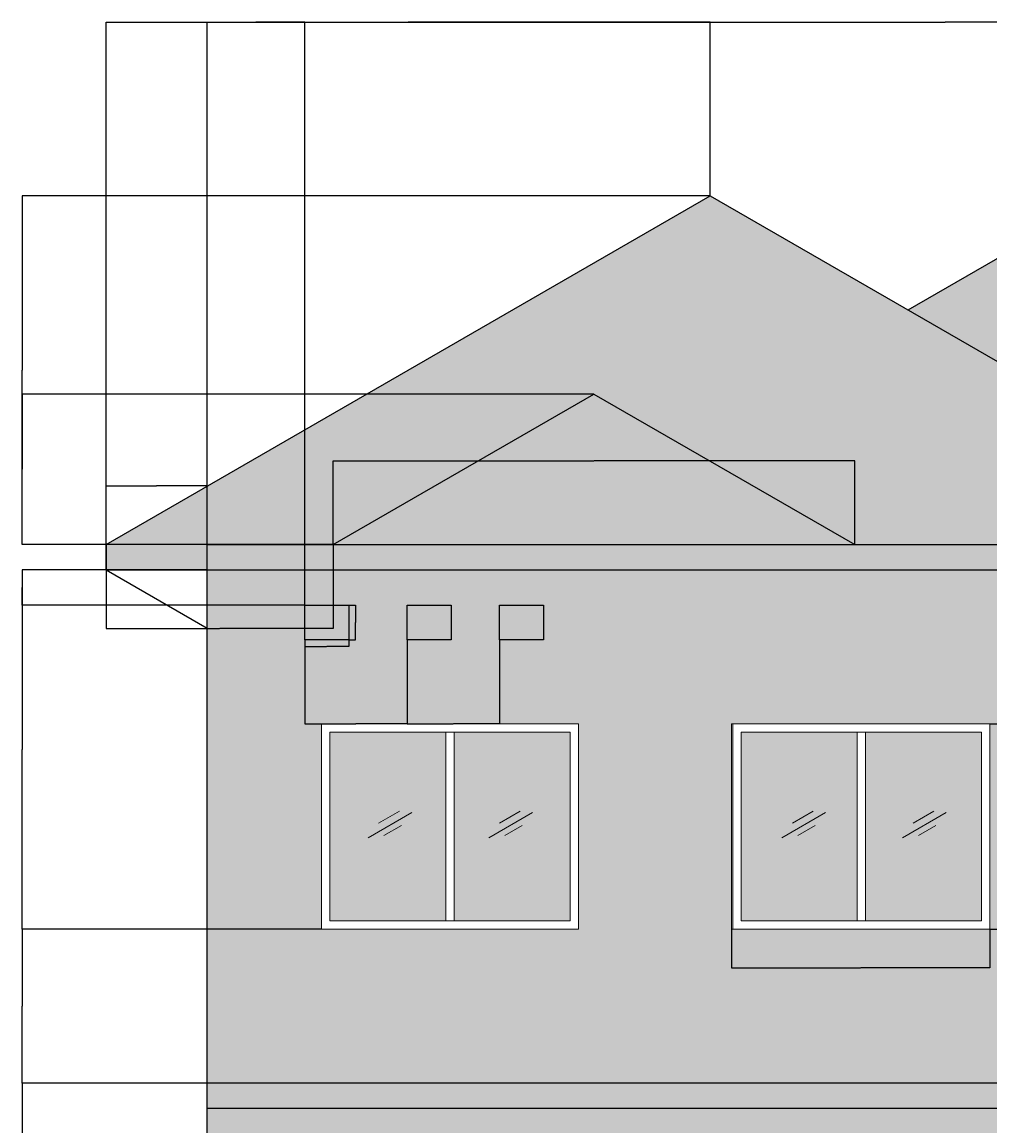
# Model space of a CAD drawing. Units: millimetres. Extents: x 2511 to 24632, y 2213 to 12972.
# Tile 4 of 5: x 13664 to 19414, y 6412 to 12972. Entities that reach past the tile are written whole.
import ezdxf

# ---------------------------------------------------------------- set-up
doc = ezdxf.new("R2010")
doc.units = ezdxf.units.MM
for name, color, linetype, lineweight in [('A-ANNO-DIMS', 2, 'Continuous', 18), ('A-ELEV', 7, 'Continuous', 25), ('A-ELEV-GLAZ', 7, 'Continuous', 18), ('A-ELEV-PATT', 13, 'Continuous', 9), ('A-ROOF', 7, 'Continuous', 25), ('A-ROOF-PATT', 13, 'Continuous', 13)]:
    doc.layers.add(name, color=color, linetype=linetype, lineweight=lineweight)
doc.layers.add('A-GLAZ-PATT', color=141, linetype='Continuous', lineweight=9, true_color=0xadddf7)
doc.styles.get("Standard").update_dxf_attribs({"font": 'arial.ttf'})
doc.dimstyles.get("Standard").update_dxf_attribs({"dimtxt": 0.18, "dimasz": 0.18, "dimexe": 0.18, "dimexo": 0.0625, "dimgap": 0.09, "dimtad": 0, "dimtih": 1, "dimtoh": 1, "dimdec": 4, "dimzin": 0, "dimdsep": 46, "dimtxsty": 'Standard', "dimcen": 0.09, "dimadec": 0, "dimazin": 0, "dimtfac": 1, "dimtdec": 4, "dimtofl": 0, "dimtmove": 0, "dimatfit": 3, "dimfxl": 1, "dimtolj": 1, "dimtzin": 0, "dimarcsym": 0})

# ---------------------------------------------------------------- blocks, each defined once
blk = doc.blocks.new('WINDOW-FRAME-1528-ELEV')
for p, q in [((3.45580574503e-05, -0.0004698816292148), (3.45580574503e-05, 1219.999530118371)), ((3.45580574503e-05, 1219.999530118371), (1527.988197152912, 1219.999530118371)), ((1527.988197152912, 1219.999530118371), (1527.988197152912, -0.0004698816292148)), ((738.9941158554847, 1169.999530118371), (738.9941158554847, 49.99953011837078)), ((788.9941158554847, 1169.999530118371), (788.9941158554847, 49.99953011837078)), ((1527.988197152912, -0.0004698816292148), (3.45580574503e-05, -0.0004698816292148))]:
    blk.add_line(p, q)
for points in [[(3.45580574503e-05, 1219.999530118371), (1527.988197152912, 1219.999530118371), (1527.988197152912, -0.0004698816292148), (3.45580574503e-05, -0.0004698816292148)], [(50.00003455805745, 1169.999530118371), (1477.988197152912, 1169.999530118371), (1477.988197152912, 49.99953011837078), (50.00003455805745, 49.99953011837078)]]:
    blk.add_lwpolyline(points, close=True)
blk = doc.blocks.new('WINDOW-FRAME-1536-ELEV')
for p, q in [((-0.0001940248657775, -0.0004698816292148), (-0.0001940248657775, 1219.999530118371)), ((-0.0001940248657775, 1219.999530118371), (1536.172544795805, 1219.999530118371)), ((1536.172544795805, 1219.999530118371), (1536.172544795805, -0.0004698816292148)), ((747.1784634983741, 1169.999530118371), (747.1784634983741, 49.99953011837078)), ((797.1784634983742, 1169.999530118371), (797.1784634983742, 49.99953011837078)), ((1536.172544795805, -0.0004698816292148), (-0.0001940248657775, -0.0004698816292148))]:
    blk.add_line(p, q)
for points in [[(8.184382200950495, 1219.999530118371), (1536.172544795805, 1219.999530118371), (1536.172544795805, -0.0004698816292148), (8.184382200950495, -0.0004698816292148)], [(58.1843822009505, 1169.999530118371), (1486.172544795805, 1169.999530118371), (1486.172544795805, 49.99953011837078), (58.1843822009505, 49.99953011837078)]]:
    blk.add_lwpolyline(points, close=True)
blk = doc.blocks.new('GLASS-REFLECTION')
for p, q in [((0.000348498528183, -0.0002333358270334), (259.2110812861792, 149.655153015964)), ((62.47510116635385, 86.0291626371336), (186.2553756901197, 157.4937374537958)), ((94.69077173755068, 13.20916119840785), (197.7341820365163, 72.70130187273116))]:
    blk.add_line(p, q)
blk = doc.blocks.new('FACADE-VENT-RECT')
blk.add_lwpolyline([(-0.0001923483068822, 206.5969172187779), (261.6107656867971, 206.5969172187779), (261.6107656867971, -0.0003445679158176), (-0.0001923483068822, -0.0003445679158176)], close=True)
blk = doc.blocks.new('*D23')
at = {"layer": 'A-ANNO-DIMS', "color": 0, "lineweight": -2, "transparency": 16777216}
for p, q in [((15342.91080765169, 9299.824155432085), (15342.91080765169, 9260.46501172682)), ((15343.09080765169, 9260.64501172682), (15472.74335351781, 9260.64501172682)), ((15604.34176568679, 9260.64501172682), (15474.68921982067, 9260.64501172682)), ((15604.52176568679, 9299.824155432085), (15604.52176568679, 9260.46501172682))]:
    blk.add_line(p, q, dxfattribs=at)
at = {"layer": 'A-ANNO-DIMS', "color": 0, "transparency": 16777216}
for points in [[(15343.09080765169, 9260.67501172682), (15343.09080765169, 9260.615011726817), (15342.91080765169, 9260.64501172682)], [(15604.34176568679, 9260.67501172682), (15604.34176568679, 9260.615011726817), (15604.52176568679, 9260.64501172682)]]:
    blk.add_solid(points, dxfattribs=at)
at = {"layer": 'Defpoints', "color": 0, "transparency": 16777216}
for p in [(15342.91080765169, 9299.886655432087), (15604.52176568679, 9299.886655432087), (15604.52176568679, 9260.64501172682)]:
    blk.add_point(p, dxfattribs=at)
at = {"layer": 'A-ANNO-DIMS', "color": 0, "transparency": 16777216, "insert": (15473.71628666924, 9260.64501172682), "char_height": 0.18, "attachment_point": 5}
blk.add_mtext('\\A1;VENT 262 TYP.', dxfattribs=at)
blk = doc.blocks.new('*D24')
at = {"layer": 'A-ANNO-DIMS', "color": 0, "lineweight": -2, "transparency": 16777216}
for p, q in [((15604.5842656868, 9506.483917218786), (15643.94340939208, 9506.483917218786)), ((15643.76340939207, 9506.303917218786), (15643.76340939207, 9403.367189463226)), ((15643.76340939207, 9300.066655432089), (15643.76340939207, 9403.003383187648)), ((15604.5842656868, 9299.886655432088), (15643.94340939208, 9299.886655432088))]:
    blk.add_line(p, q, dxfattribs=at)
at = {"layer": 'A-ANNO-DIMS', "color": 0, "transparency": 16777216}
for points in [[(15643.73340939208, 9506.303917218786), (15643.79340939208, 9506.303917218786), (15643.76340939207, 9506.483917218786)], [(15643.73340939208, 9300.066655432089), (15643.79340939208, 9300.066655432089), (15643.76340939207, 9299.886655432088)]]:
    blk.add_solid(points, dxfattribs=at)
at = {"layer": 'Defpoints', "color": 0, "transparency": 16777216}
for p in [(15604.5217656868, 9506.483917218786), (15643.76340939207, 9506.483917218786), (15604.5217656868, 9299.886655432088)]:
    blk.add_point(p, dxfattribs=at)
at = {"layer": 'A-ANNO-DIMS', "color": 0, "transparency": 16777216, "insert": (15643.76340939207, 9403.18528632543), "char_height": 0.18, "attachment_point": 5}
blk.add_mtext('\\A1;207 TYP.', dxfattribs=at)
blk = doc.blocks.new('*D33')
at = {"layer": 'A-ANNO-DIMS', "color": 0, "lineweight": -2, "transparency": 16777216}
for p, q in [((17877.81880597513, 7581.154030118369), (17877.81880597513, 7350.610619295268)), ((19413.9915447958, 7581.154030118369), (19413.9915447958, 7350.610619295268)), ((17877.99880597513, 7350.790619295269), (18644.76734455327, 7350.790619295269)), ((19413.8115447958, 7350.790619295269), (18647.04300621766, 7350.790619295269))]:
    blk.add_line(p, q, dxfattribs=at)
at = {"layer": 'A-ANNO-DIMS', "color": 0, "transparency": 16777216}
for points in [[(17877.99880597513, 7350.820619295268), (17877.99880597513, 7350.760619295269), (17877.81880597513, 7350.790619295269)], [(19413.8115447958, 7350.820619295268), (19413.8115447958, 7350.760619295269), (19413.9915447958, 7350.790619295269)]]:
    blk.add_solid(points, dxfattribs=at)
at = {"layer": 'Defpoints', "color": 0, "transparency": 16777216}
for p in [(17877.81880597513, 7581.21653011837), (19413.9915447958, 7581.21653011837), (19413.9915447958, 7350.790619295269)]:
    blk.add_point(p, dxfattribs=at)
at = {"layer": 'A-ANNO-DIMS', "color": 0, "transparency": 16777216, "insert": (18645.90517538547, 7350.790619295269), "char_height": 0.18, "attachment_point": 5}
blk.add_mtext('\\A1;FRAME 1536 TYP.', dxfattribs=at)
blk = doc.blocks.new('*D34')
at = {"layer": 'A-ANNO-DIMS', "color": 0, "lineweight": -2, "transparency": 16777216}
for p, q in [((19414.05404479581, 8801.216530118374), (19644.59745561891, 8801.216530118374)), ((19644.41745561891, 8801.036530118374), (19644.41745561892, 8191.398433256164)), ((19644.41745561892, 7581.396530118374), (19644.41745561892, 8191.034626980584)), ((19414.05404479581, 7581.216530118374), (19644.59745561892, 7581.216530118374))]:
    blk.add_line(p, q, dxfattribs=at)
at = {"layer": 'A-ANNO-DIMS', "color": 0, "transparency": 16777216}
for points in [[(19644.38745561891, 8801.036530118374), (19644.44745561891, 8801.036530118374), (19644.41745561891, 8801.216530118374)], [(19644.38745561892, 7581.396530118374), (19644.44745561891, 7581.396530118374), (19644.41745561892, 7581.216530118374)]]:
    blk.add_solid(points, dxfattribs=at)
at = {"layer": 'Defpoints', "color": 0, "transparency": 16777216}
for p in [(19413.99154479581, 8801.216530118374), (19644.41745561891, 8801.216530118374), (19413.99154479581, 7581.216530118374)]:
    blk.add_point(p, dxfattribs=at)
at = {"layer": 'A-ANNO-DIMS', "color": 0, "transparency": 16777216, "insert": (19644.41745561891, 8191.216530118365), "char_height": 0.18, "attachment_point": 5}
blk.add_mtext('\\A1;1220 TYP.', dxfattribs=at)
blk = doc.blocks.new('*D64')
at = {"layer": 'A-ANNO-DIMS', "color": 0, "lineweight": -2, "transparency": 16777216}
for p, q in [((14162.809797, 9866.279030000002), (14162.809797, 12971.685584)), ((14162.989797, 12971.505584), (19147.45133178854, 12971.505584)), ((24132.629797, 12971.505584), (19148.16826221146, 12971.505584)), ((24132.809797, 9716.27903), (24132.809797, 12971.685584))]:
    blk.add_line(p, q, dxfattribs=at)
at = {"layer": 'A-ANNO-DIMS', "color": 0, "transparency": 16777216}
for points in [[(14162.989797, 12971.535584), (14162.989797, 12971.475584), (14162.809797, 12971.505584)], [(24132.629797, 12971.535584), (24132.629797, 12971.475584), (24132.809797, 12971.505584)]]:
    blk.add_solid(points, dxfattribs=at)
at = {"layer": 'Defpoints', "color": 0, "transparency": 16777216}
for p in [(14162.809797, 12971.505584), (14162.809797, 9866.21653), (24132.809797, 9716.21653)]:
    blk.add_point(p, dxfattribs=at)
at = {"layer": 'A-ANNO-DIMS', "color": 0, "transparency": 16777216, "insert": (19147.809797, 12971.505584), "char_height": 0.18, "attachment_point": 5}
blk.add_mtext('\\A1;9970', dxfattribs=at)
blk = doc.blocks.new('*D68')
at = {"layer": 'A-ANNO-DIMS', "color": 0, "lineweight": -2, "transparency": 16777216}
for p, q in [((14762.747297, 6666.216530000004), (13663.87979700001, 6666.216530000003)), ((13664.05979700001, 6666.036530000003), (13664.05979700001, 5523.898433137791)), ((13664.05979700001, 4381.39653), (13664.05979700001, 5523.534626862211)), ((15441.75253500001, 4381.216530000002), (13663.87979700001, 4381.21653))]:
    blk.add_line(p, q, dxfattribs=at)
at = {"layer": 'A-ANNO-DIMS', "color": 0, "transparency": 16777216}
for points in [[(13664.02979700001, 6666.036530000003), (13664.08979700001, 6666.036530000003), (13664.05979700001, 6666.216530000003)], [(13664.02979700001, 4381.39653), (13664.08979700001, 4381.39653), (13664.05979700001, 4381.21653)]]:
    blk.add_solid(points, dxfattribs=at)
at = {"layer": 'Defpoints', "color": 0, "transparency": 16777216}
for p in [(13664.05979700001, 6666.216530000003), (14762.809797, 6666.216530000004), (15441.81503500001, 4381.216530000002)]:
    blk.add_point(p, dxfattribs=at)
at = {"layer": 'A-ANNO-DIMS', "color": 0, "transparency": 16777216, "insert": (13664.05979700001, 5523.716529999997), "char_height": 0.18, "attachment_point": 5}
blk.add_mtext('\\A1;2285', dxfattribs=at)
blk = doc.blocks.new('*D69')
at = {"layer": 'A-ANNO-DIMS', "color": 0, "lineweight": -2, "transparency": 16777216}
for p, q in [((15441.75253500001, 7581.216530000003), (13663.87979700001, 7581.216530000003)), ((13664.05979700001, 7581.036530000003), (13664.05979700001, 7123.898433137792)), ((13664.05979700001, 6666.396530000003), (13664.05979700001, 7123.534626862213)), ((14762.747297, 6666.216530000004), (13663.87979700001, 6666.216530000003))]:
    blk.add_line(p, q, dxfattribs=at)
at = {"layer": 'A-ANNO-DIMS', "color": 0, "transparency": 16777216}
for points in [[(13664.02979700001, 7581.036530000003), (13664.08979700001, 7581.036530000003), (13664.05979700001, 7581.216530000003)], [(13664.02979700001, 6666.396530000003), (13664.08979700001, 6666.396530000003), (13664.05979700001, 6666.216530000003)]]:
    blk.add_solid(points, dxfattribs=at)
at = {"layer": 'Defpoints', "color": 0, "transparency": 16777216}
for p in [(13664.05979700001, 7581.216530000003), (15441.81503500001, 7581.216530000003), (14762.809797, 6666.216530000004)]:
    blk.add_point(p, dxfattribs=at)
at = {"layer": 'A-ANNO-DIMS', "color": 0, "transparency": 16777216, "insert": (13664.05979700001, 7123.716529999997), "char_height": 0.18, "attachment_point": 5}
blk.add_mtext('\\A1;915', dxfattribs=at)
blk = doc.blocks.new('*D70')
at = {"layer": 'A-ANNO-DIMS', "color": 0, "lineweight": -2, "transparency": 16777216}
for p, q in [((14762.747297, 9716.216530000003), (13663.87979700001, 9716.216530000003)), ((13664.05979700001, 9716.036530000003), (13664.05979700001, 8648.898494529332)), ((13664.05979700001, 7581.396530000003), (13664.05979700001, 8648.534565470674)), ((15441.75253500001, 7581.216530000003), (13663.87979700001, 7581.216530000003))]:
    blk.add_line(p, q, dxfattribs=at)
at = {"layer": 'A-ANNO-DIMS', "color": 0, "transparency": 16777216}
for points in [[(13664.02979700001, 9716.036530000003), (13664.08979700001, 9716.036530000003), (13664.05979700001, 9716.216530000003)], [(13664.02979700001, 7581.396530000003), (13664.08979700001, 7581.396530000003), (13664.05979700001, 7581.216530000003)]]:
    blk.add_solid(points, dxfattribs=at)
at = {"layer": 'Defpoints', "color": 0, "transparency": 16777216}
for p in [(13664.05979700001, 9716.216530000003), (14762.809797, 9716.216530000003), (15441.81503500001, 7581.216530000003)]:
    blk.add_point(p, dxfattribs=at)
at = {"layer": 'A-ANNO-DIMS', "color": 0, "transparency": 16777216, "insert": (13664.05979700001, 8648.71653), "char_height": 0.18, "attachment_point": 5}
blk.add_mtext('\\A1;2135', dxfattribs=at)
blk = doc.blocks.new('*D82')
at = {"layer": 'A-ANNO-DIMS', "color": 0, "lineweight": -2, "transparency": 16777216}
for p, q in [((14162.809797, 9716.27903), (14162.809797, 10215.14653)), ((14162.989797, 10214.96653), (14462.5207656221, 10214.96653)), ((14762.629797, 10214.96653), (14463.0988283779, 10214.96653)), ((14762.809797, 9716.27903), (14762.809797, 10215.14653))]:
    blk.add_line(p, q, dxfattribs=at)
at = {"layer": 'A-ANNO-DIMS', "color": 0, "transparency": 16777216}
for points in [[(14162.989797, 10214.99653), (14162.989797, 10214.93653), (14162.809797, 10214.96653)], [(14762.629797, 10214.99653), (14762.629797, 10214.93653), (14762.809797, 10214.96653)]]:
    blk.add_solid(points, dxfattribs=at)
at = {"layer": 'Defpoints', "color": 0, "transparency": 16777216}
for p in [(14762.809797, 10214.96653), (14162.809797, 9716.21653), (14762.809797, 9716.21653)]:
    blk.add_point(p, dxfattribs=at)
at = {"layer": 'A-ANNO-DIMS', "color": 0, "transparency": 16777216, "insert": (14462.809797, 10214.96653), "char_height": 0.18, "attachment_point": 5}
blk.add_mtext('\\A1;600', dxfattribs=at)
blk = doc.blocks.new('*D84')
at = {"layer": 'A-ANNO-DIMS', "color": 0, "lineweight": -2, "transparency": 16777216}
for p, q in [((15950.742303, 9299.824155), (15950.742303, 8800.956655)), ((16500.795593, 9299.824155), (16500.795593, 8800.956655)), ((15950.922303, 8801.136655), (16225.48040775443, 8801.136655)), ((16500.615593, 8801.136655), (16226.05748824557, 8801.136655))]:
    blk.add_line(p, q, dxfattribs=at)
at = {"layer": 'A-ANNO-DIMS', "color": 0, "transparency": 16777216}
for points in [[(15950.922303, 8801.166655), (15950.922303, 8801.106655), (15950.742303, 8801.136655)], [(16500.615593, 8801.166655), (16500.615593, 8801.106655), (16500.795593, 8801.136655)]]:
    blk.add_solid(points, dxfattribs=at)
at = {"layer": 'Defpoints', "color": 0, "transparency": 16777216}
for p in [(15950.742303, 9299.886654999998), (16500.795593, 9299.886654999998), (15950.742303, 8801.136655)]:
    blk.add_point(p, dxfattribs=at)
at = {"layer": 'A-ANNO-DIMS', "color": 0, "transparency": 16777216, "insert": (16225.768948, 8801.136655), "char_height": 0.18, "attachment_point": 5}
blk.add_mtext('\\A1;550', dxfattribs=at)
blk = doc.blocks.new('*D85')
at = {"layer": 'A-ANNO-DIMS', "color": 0, "lineweight": -2, "transparency": 16777216}
for p, q in [((15342.910808, 9299.824155), (15342.910808, 8800.956655)), ((15950.742303, 9299.824155), (15950.742303, 8800.956655)), ((15343.090808, 8801.136655), (15646.4321762367, 8801.136655)), ((15950.562303, 8801.136655), (15647.2209347633, 8801.136655))]:
    blk.add_line(p, q, dxfattribs=at)
at = {"layer": 'A-ANNO-DIMS', "color": 0, "transparency": 16777216}
for points in [[(15343.090808, 8801.166655), (15343.090808, 8801.106655), (15342.910808, 8801.136655)], [(15950.562303, 8801.166655), (15950.562303, 8801.106655), (15950.742303, 8801.136655)]]:
    blk.add_solid(points, dxfattribs=at)
at = {"layer": 'Defpoints', "color": 0, "transparency": 16777216}
for p in [(15342.910808, 9299.886654999998), (15950.742303, 9299.886654999998), (15342.910808, 8801.136655)]:
    blk.add_point(p, dxfattribs=at)
at = {"layer": 'A-ANNO-DIMS', "color": 0, "transparency": 16777216, "insert": (15646.8265555, 8801.136655), "char_height": 0.18, "attachment_point": 5}
blk.add_mtext('\\A1;607.8', dxfattribs=at)
blk = doc.blocks.new('*D86')
at = {"layer": 'A-ANNO-DIMS', "color": 0, "lineweight": -2, "transparency": 16777216}
for p, q in [((14762.809797, 9716.27903), (14762.809797, 12971.685584)), ((14762.989797, 12971.505584), (15052.48397234993, 12971.505584)), ((15342.730808, 12971.505584), (15053.23663265007, 12971.505584)), ((15342.910808, 9506.546417), (15342.910808, 12971.685584))]:
    blk.add_line(p, q, dxfattribs=at)
at = {"layer": 'A-ANNO-DIMS', "color": 0, "transparency": 16777216}
for points in [[(14762.989797, 12971.535584), (14762.989797, 12971.475584), (14762.809797, 12971.505584)], [(15342.730808, 12971.535584), (15342.730808, 12971.475584), (15342.910808, 12971.505584)]]:
    blk.add_solid(points, dxfattribs=at)
at = {"layer": 'Defpoints', "color": 0, "transparency": 16777216}
for p in [(15342.910808, 12971.505584), (14762.809797, 9716.21653), (15342.910808, 9506.483917)]:
    blk.add_point(p, dxfattribs=at)
at = {"layer": 'A-ANNO-DIMS', "color": 0, "transparency": 16777216, "insert": (15052.8603025, 12971.505584), "char_height": 0.18, "attachment_point": 5}
blk.add_mtext('\\A1;580.1', dxfattribs=at)
blk = doc.blocks.new('*D87')
at = {"layer": 'A-ANNO-DIMS', "color": 0, "lineweight": -2, "transparency": 16777216}
for p, q in [((14762.747297, 9716.216530000003), (13663.87979700001, 9716.216530000003)), ((13664.05979700001, 9716.036530000003), (13664.05979700001, 9611.532188029334)), ((13664.05979700001, 9506.663917000002), (13664.05979700001, 9611.168258970672)), ((15342.848308, 9506.483917000001), (13663.87979700001, 9506.483917000001))]:
    blk.add_line(p, q, dxfattribs=at)
at = {"layer": 'A-ANNO-DIMS', "color": 0, "transparency": 16777216}
for points in [[(13664.02979700001, 9716.036530000003), (13664.08979700001, 9716.036530000003), (13664.05979700001, 9716.216530000003)], [(13664.02979700001, 9506.663917000002), (13664.08979700001, 9506.663917000002), (13664.05979700001, 9506.483917000001)]]:
    blk.add_solid(points, dxfattribs=at)
at = {"layer": 'Defpoints', "color": 0, "transparency": 16777216}
for p in [(14762.809797, 9716.216530000003), (13664.05979700001, 9506.483917000001), (15342.910808, 9506.483917000001)]:
    blk.add_point(p, dxfattribs=at)
at = {"layer": 'A-ANNO-DIMS', "color": 0, "transparency": 16777216, "insert": (13664.05979700001, 9611.350223499998), "char_height": 0.18, "attachment_point": 5}
blk.add_mtext('\\A1;209.73', dxfattribs=at)
blk = doc.blocks.new('*D88')
at = {"layer": 'A-ANNO-DIMS', "color": 0, "lineweight": -2, "transparency": 16777216}
for p, q in [((17752.200329, 11938.588205), (13663.87979700001, 11938.588205)), ((13664.05979700001, 11938.408205), (13664.05979700001, 10902.58427063779)), ((13664.05979700001, 9866.396530000004), (13664.05979700001, 10902.22046436221)), ((14162.747297, 9866.216530000003), (13663.87979700001, 9866.216530000003))]:
    blk.add_line(p, q, dxfattribs=at)
at = {"layer": 'A-ANNO-DIMS', "color": 0, "transparency": 16777216}
for points in [[(13664.02979700001, 11938.408205), (13664.08979700001, 11938.408205), (13664.05979700001, 11938.588205)], [(13664.02979700001, 9866.396530000004), (13664.08979700001, 9866.396530000004), (13664.05979700001, 9866.216530000003)]]:
    blk.add_solid(points, dxfattribs=at)
at = {"layer": 'Defpoints', "color": 0, "transparency": 16777216}
for p in [(13664.05979700001, 11938.588205), (17752.262829, 11938.588205), (14162.80979700001, 9866.216530000003)]:
    blk.add_point(p, dxfattribs=at)
at = {"layer": 'A-ANNO-DIMS', "color": 0, "transparency": 16777216, "insert": (13664.05979700001, 10902.4023675), "char_height": 0.18, "attachment_point": 5}
blk.add_mtext('\\A1;2072.4', dxfattribs=at)
blk = doc.blocks.new('*D90')
at = {"layer": 'A-ANNO-DIMS', "color": 0, "lineweight": -2, "transparency": 16777216}
for p, q in [((14162.809797, 9866.279030000002), (14162.809797, 12971.685584)), ((14162.989797, 12971.505584), (15957.07207016235, 12971.505584)), ((17752.082829, 12971.505584), (15958.00055583765, 12971.505584)), ((17752.262829, 11938.650705), (17752.262829, 12971.685584))]:
    blk.add_line(p, q, dxfattribs=at)
at = {"layer": 'A-ANNO-DIMS', "color": 0, "transparency": 16777216}
for points in [[(14162.989797, 12971.535584), (14162.989797, 12971.475584), (14162.809797, 12971.505584)], [(17752.082829, 12971.535584), (17752.082829, 12971.475584), (17752.262829, 12971.505584)]]:
    blk.add_solid(points, dxfattribs=at)
at = {"layer": 'Defpoints', "color": 0, "transparency": 16777216}
for p in [(17752.262829, 12971.505584), (17752.262829, 11938.588205), (14162.809797, 9866.21653)]:
    blk.add_point(p, dxfattribs=at)
at = {"layer": 'A-ANNO-DIMS', "color": 0, "transparency": 16777216, "insert": (15957.536313, 12971.505584), "char_height": 0.18, "attachment_point": 5}
blk.add_mtext('\\A1;3589.5', dxfattribs=at)
blk = doc.blocks.new('*D91')
at = {"layer": 'A-ANNO-DIMS', "color": 0, "lineweight": -2, "transparency": 16777216}
for p, q in [((15511.626108, 9866.279030000002), (15511.626108, 10365.14653)), ((18611.109928, 9866.279030000002), (18611.109928, 10365.14653)), ((15511.806108, 10364.96653), (17060.90377516235, 10364.96653)), ((18610.929928, 10364.96653), (17061.83226083765, 10364.96653))]:
    blk.add_line(p, q, dxfattribs=at)
at = {"layer": 'A-ANNO-DIMS', "color": 0, "transparency": 16777216}
for points in [[(15511.806108, 10364.99653), (15511.806108, 10364.93653), (15511.626108, 10364.96653)], [(18610.929928, 10364.99653), (18610.929928, 10364.93653), (18611.109928, 10364.96653)]]:
    blk.add_solid(points, dxfattribs=at)
at = {"layer": 'Defpoints', "color": 0, "transparency": 16777216}
for p in [(18611.109928, 10364.96653), (15511.626108, 9866.21653), (18611.109928, 9866.21653)]:
    blk.add_point(p, dxfattribs=at)
at = {"layer": 'A-ANNO-DIMS', "color": 0, "transparency": 16777216, "insert": (17061.368018, 10364.96653), "char_height": 0.18, "attachment_point": 5}
blk.add_mtext('\\A1;3099.5', dxfattribs=at)
blk = doc.blocks.new('*D92')
at = {"layer": 'A-ANNO-DIMS', "color": 0, "lineweight": -2, "transparency": 16777216}
for p, q in [((14162.809797, 9866.15403), (14162.809797, 9367.28653)), ((15511.626108, 9866.15403), (15511.626108, 9367.28653)), ((14162.989797, 9367.46653), (14836.76261143588, 9367.46653)), ((15511.446108, 9367.46653), (14837.67329356412, 9367.46653))]:
    blk.add_line(p, q, dxfattribs=at)
at = {"layer": 'A-ANNO-DIMS', "color": 0, "transparency": 16777216}
for points in [[(14162.989797, 9367.496530000002), (14162.989797, 9367.436529999999), (14162.809797, 9367.46653)], [(15511.446108, 9367.496530000002), (15511.446108, 9367.436529999999), (15511.626108, 9367.46653)]]:
    blk.add_solid(points, dxfattribs=at)
at = {"layer": 'Defpoints', "color": 0, "transparency": 16777216}
for p in [(14162.809797, 9866.21653), (15511.626108, 9866.21653), (14162.809797, 9367.46653)]:
    blk.add_point(p, dxfattribs=at)
at = {"layer": 'A-ANNO-DIMS', "color": 0, "transparency": 16777216, "insert": (14837.2179525, 9367.46653), "char_height": 0.18, "attachment_point": 5}
blk.add_mtext('\\A1;1348.8', dxfattribs=at)
blk = doc.blocks.new('*D93')
at = {"layer": 'A-ANNO-DIMS', "color": 0, "lineweight": -2, "transparency": 16777216}
for p, q in [((17061.30551800001, 10760.960439), (13663.87979700001, 10760.960439)), ((13664.05979700001, 10760.780439), (13664.05979700001, 10313.77038763779)), ((13664.05979700001, 9866.396530000004), (13664.05979700001, 10313.40658136221)), ((15511.56360800001, 9866.216530000003), (13663.87979700001, 9866.216530000003))]:
    blk.add_line(p, q, dxfattribs=at)
at = {"layer": 'A-ANNO-DIMS', "color": 0, "transparency": 16777216}
for points in [[(13664.02979700001, 10760.780439), (13664.08979700001, 10760.780439), (13664.05979700001, 10760.960439)], [(13664.02979700001, 9866.396530000004), (13664.08979700001, 9866.396530000004), (13664.05979700001, 9866.216530000003)]]:
    blk.add_solid(points, dxfattribs=at)
at = {"layer": 'Defpoints', "color": 0, "transparency": 16777216}
for p in [(17061.36801800001, 10760.960439), (13664.05979700001, 9866.216530000003), (15511.626108, 9866.216530000003)]:
    blk.add_point(p, dxfattribs=at)
at = {"layer": 'A-ANNO-DIMS', "color": 0, "transparency": 16777216, "insert": (13664.05979700001, 10313.5884845), "char_height": 0.18, "attachment_point": 5}
blk.add_mtext('\\A1;894.7', dxfattribs=at)

msp = doc.modelspace()

# ---------------------------------------------------------------- hatches: boundary and pattern name
at = {"layer": 'A-ELEV-PATT', "transparency": 33554551}
h = msp.add_hatch(color=256, dxfattribs=at)
h.dxf.hatch_style = 1
h.paths.add_polyline_path([(20858.80979657499, 6516.216530118374), (14762.80979657499, 6516.21653011837), (14762.80979657499, 3466.216530118371), (19843.80979657499, 3466.216530118371), (19843.80979657499, 5601.216530118371), (20718.80979657499, 5601.216530118371), (20718.80979657499, 3466.216530118371), (20858.80979657499, 3466.216530118371)])
h.paths.add_polyline_path([(16969.80319715291, 5601.216530118371), (16969.80319715291, 4381.21653011837), (15441.81503455806, 4381.21653011837), (15441.81503455806, 5601.216530118371)], flags=16)
h.paths.add_polyline_path([(16919.80319715291, 5551.21653011837), (16919.80319715291, 4431.21653011837), (15491.81503455806, 4431.21653011837), (15491.81503455806, 5551.21653011837)], flags=0)
h.paths.add_polyline_path([(17877.81880597513, 5601.216530118371), (19413.9915447958, 5601.216530118371), (19413.9915447958, 4381.21653011837), (17886.00338220095, 4381.21653011837), (17877.81880597513, 4381.21653011837)], flags=16)
h.paths.add_polyline_path([(17936.00338220095, 5551.21653011837), (19363.9915447958, 5551.21653011837), (19363.9915447958, 4431.21653011837), (17936.00338220095, 4431.21653011837)], flags=0)
h.paths.add_polyline_path([(20858.80979657499, 9716.216530118376), (14762.80979657499, 9716.21653011837), (14762.80979657499, 6666.21653011837), (19522.169078361, 6666.21653011837), (19522.169078361, 7733.216530118371), (20858.80979657499, 7733.216530118371)])
h.paths.add_polyline_path([(16969.80319715291, 8801.21653011837), (16969.80319715291, 7581.216530118371), (15441.81503455806, 7581.216530118371), (15441.81503455806, 8801.21653011837)], flags=16)
h.paths.add_polyline_path([(16919.80319715291, 8751.216530118369), (16919.80319715291, 7631.216530118371), (15491.81503455806, 7631.216530118371), (15491.81503455806, 8751.216530118369)], flags=0)
h.paths.add_polyline_path([(17877.81880597514, 8801.21653011837), (19413.9915447958, 8801.21653011837), (19413.9915447958, 7581.216530118371), (17886.00338220095, 7581.216530118371), (17877.81880597513, 7581.216530118371)], flags=16)
h.paths.add_polyline_path([(17936.00338220095, 8751.216530118369), (19363.9915447958, 8751.216530118369), (19363.9915447958, 7631.216530118371), (17936.00338220095, 7631.216530118371)], flags=0)
h.paths.add_polyline_path([(23051.60643531334, 9716.216530118376), (20858.80979657499, 9716.21653011837), (20858.80979657499, 7733.216530118371), (23051.60643531334, 7733.216530118371)])
h.paths.add_polyline_path([(23051.60643531335, 6516.216530118374), (20858.80979657499, 6516.216530118374), (20858.80979657499, 3516.21653011837), (23051.60643531335, 3516.21653011837)])
h = msp.add_hatch(color=256, dxfattribs=at)
h.dxf.hatch_style = 1
h.paths.add_polyline_path([(23708.80979657499, 6666.21653011837), (14762.80979657499, 6666.21653011837), (14762.80979657499, 6516.21653011837), (23708.80979657499, 6516.216530118374)])
at = {"layer": 'A-GLAZ-PATT'}
h = msp.add_hatch(color=256, dxfattribs=at)
h.dxf.hatch_style = 1
h.paths.add_polyline_path([(16180.80911585549, 8751.216530118369), (15491.81503455806, 8751.216530118369), (15491.81503455806, 7631.216530118371), (16180.80911585549, 7631.216530118371)])
h.paths.add_polyline_path([(16919.80319715291, 8751.216530118369), (16230.80911585548, 8751.216530118369), (16230.80911585548, 7631.216530118371), (16919.80319715291, 7631.216530118371)])
h.paths.add_polyline_path([(18624.99746349838, 8751.216530118369), (17936.00338220095, 8751.216530118369), (17936.00338220095, 7631.216530118371), (18624.99746349838, 7631.216530118371)])
h.paths.add_polyline_path([(19363.9915447958, 8751.216530118369), (18674.99746349837, 8751.216530118369), (18674.99746349837, 7631.216530118371), (19363.9915447958, 7631.216530118371)])
h.paths.add_polyline_path([(16180.80911585548, 5551.21653011837), (15491.81503455806, 5551.21653011837), (15491.81503455806, 4431.21653011837), (16180.80911585548, 4431.21653011837)])
h.paths.add_polyline_path([(16919.80319715291, 5551.21653011837), (16230.80911585548, 5551.21653011837), (16230.80911585548, 4431.21653011837), (16919.80319715291, 4431.21653011837)])
h.paths.add_polyline_path([(18624.99746349837, 5551.21653011837), (17936.00338220095, 5551.21653011837), (17936.00338220095, 4431.21653011837), (18624.99746349837, 4431.21653011837)])
h.paths.add_polyline_path([(19363.9915447958, 5551.21653011837), (18674.99746349837, 5551.21653011837), (18674.99746349837, 4431.21653011837), (19363.9915447958, 4431.21653011837)])
at = {"layer": 'A-ROOF-PATT'}
h = msp.add_hatch(dxfattribs=at)
h.set_pattern_fill('ANGLE', color=256, scale=15)
h.set_pattern_definition([(0, (11792.595132882, -12295.09862892571), (0, 104.775), [76.2, -28.575]), (90, (11792.595132882, -12295.09862892571), (-104.775, 6.4e-15), [76.2, -28.575])])
h.paths.add_polyline_path([(17752.26282908254, 11938.58820468012), (14162.80979657499, 9866.216530118376), (14762.80979657499, 9866.216530118376), (15511.62610781541, 9866.216530118376), (17061.36801812783, 10760.96043921169), (18611.10992844025, 9866.216530118376), (21341.71586159009, 9866.21653011837)])
h.paths.add_polyline_path([(21026.45751448832, 12472.755584324), (18926.75765114087, 11260.49330300292), (21341.71586159008, 9866.21653011837), (23532.80979657499, 9866.21653011837), (24132.80979657499, 9866.21653011837)])
h.paths.add_polyline_path([(17061.36801812783, 10760.96043921169), (15511.62610781541, 9866.216530118376), (18611.10992844025, 9866.21653011837)], flags=17)
at = {"layer": 'A-ROOF-PATT', "transparency": 33554551}
h = msp.add_hatch(color=256, dxfattribs=at)
h.dxf.hatch_style = 1
h.paths.add_polyline_path([(24132.80979657499, 9866.21653011837), (23532.80979657499, 9866.21653011837), (14762.80979657499, 9866.216530118376), (14162.80979657499, 9866.216530118376), (14162.80979657499, 9716.21653011837), (14762.80979657499, 9716.21653011837), (23532.80979657499, 9716.216530118376), (24132.80979657499, 9716.216530118376)])

# ---------------------------------------------------------------- linework, layer by layer
at = {"layer": 'A-ELEV'}
for p, q in [((14762.80979657499, 6666.21653011837), (14762.80979657499, 9716.216530118376)), ((14762.80979657499, 3466.216530118371), (14762.80979657499, 7733.216530118371)), ((23708.80979657499, 6666.21653011837), (14762.80979657499, 6666.21653011837)), ((14762.80979657499, 6516.21653011837), (23708.80979657499, 6516.216530118374))]:
    msp.add_line(p, q, dxfattribs=at)
at = {"layer": 'A-ROOF'}
for p, q in [((21026.45751448832, 12472.755584324), (18926.75765114087, 11260.49330300292)), ((14162.80979657499, 9866.216530118376), (17752.26282908254, 11938.58820468012)), ((17752.26282908254, 11938.58820468012), (21341.71586159009, 9866.21653011837)), ((15511.62610781541, 9866.216530118376), (17061.36801812783, 10760.96043921169)), ((17061.36801812783, 10760.96043921169), (18611.10992844024, 9866.216530118376)), ((14762.80979657499, 9866.216530118376), (14162.80979657499, 9866.216530118376)), ((14162.80979657499, 9866.216530118376), (14162.80979657499, 9716.21653011837)), ((14762.80979657499, 9866.216530118376), (23532.80979657499, 9866.21653011837)), ((14162.80979657499, 9716.21653011837), (14762.80979657499, 9716.21653011837)), ((14162.80979657499, 9716.21653011837), (14762.80979657499, 9369.806368604599)), ((14762.80979657499, 9716.21653011837), (23532.80979657499, 9716.216530118376))]:
    msp.add_line(p, q, dxfattribs=at)

# ---------------------------------------------------------------- block references
at = {"layer": 'A-ELEV'}
for p in [(15342.911, 9299.887), (15950.74249530715, 9299.887), (16500.79578584541, 9299.887)]:
    msp.add_blockref('FACADE-VENT-RECT', p, dxfattribs=at)
at = {"layer": 'A-ELEV-GLAZ'}
for name, p in [('WINDOW-FRAME-1528-ELEV', (15441.815, 7581.216999999999)), ('WINDOW-FRAME-1536-ELEV', (17877.819, 7581.216999999999)), ('GLASS-REFLECTION', (15719.254, 8124.306999999999)), ('GLASS-REFLECTION', (16437.39000946567, 8124.306999999999)), ('GLASS-REFLECTION', (18178.49078937554, 8124.306999999999)), ('GLASS-REFLECTION', (18894.90375053235, 8124.306999999999))]:
    msp.add_blockref(name, p, dxfattribs=at)

# ---------------------------------------------------------------- dimensions: what is measured, and where the dimension line sits
at = {"layer": 'A-ANNO-DIMS'}
for base, p1, p2, override, picture, middle in [((14162.809797, 12971.505584), (24132.809797, 9716.21653), (14162.809797, 9866.21653), {"dimdec": 0, "dimlfac": 1, "dimrnd": 0, "dimzin": 0, "dimdsep": 46, "dimlunit": 2}, '*D64', (19147.809797, 12971.505584)), ((17752.262829, 12971.505584), (14162.809797, 9866.21653), (17752.262829, 11938.588205), {"dimdec": 1, "dimlfac": 1, "dimrnd": 0, "dimzin": 0, "dimdsep": 46, "dimlunit": 2}, '*D90', (15957.536313, 12971.505584)), ((15342.910808, 12971.505584), (14762.809797, 9716.21653), (15342.910808, 9506.483917), {"dimdec": 1, "dimlfac": 1, "dimrnd": 0, "dimzin": 0, "dimdsep": 46, "dimlunit": 2}, '*D86', (15052.8603025, 12971.505584)), ((18611.109928, 10364.96653), (15511.626108, 9866.21653), (18611.109928, 9866.21653), {"dimdec": 1, "dimlfac": 1, "dimrnd": 0, "dimzin": 0, "dimdsep": 46, "dimlunit": 2}, '*D91', (17061.368018, 10364.96653)), ((14762.809797, 10214.96653), (14162.809797, 9716.21653), (14762.809797, 9716.21653), {"dimdec": 0, "dimlfac": 1, "dimrnd": 0, "dimzin": 0, "dimdsep": 46, "dimlunit": 2}, '*D82', (14462.809797, 10214.96653))]:
    dim = msp.add_linear_dim(base=base, p1=p1, p2=p2, dimstyle='Standard', override=override, dxfattribs=at)
    dim.commit()
    dim.dimension.update_dxf_attribs({"geometry": picture, "text_midpoint": middle})
for base, p1, p2, angle, override, picture, middle in [((13664.05979700001, 11938.588205), (14162.809797, 9866.21653), (17752.262829, 11938.588205), 90, {"dimdec": 1, "dimlfac": 1, "dimrnd": 0, "dimzin": 0, "dimdsep": 46, "dimlunit": 2}, '*D88', (13664.05979700001, 10902.4023675)), ((13664.05979700001, 9866.216530000003), (17061.368018, 10760.960439), (15511.626108, 9866.21653), 90, {"dimdec": 1, "dimlfac": 1, "dimrnd": 0, "dimzin": 0, "dimdsep": 46, "dimlunit": 2}, '*D93', (13664.05979700001, 10313.5884845)), ((14162.809797, 9367.46653), (15511.626108, 9866.21653), (14162.809797, 9866.21653), 180, {"dimdec": 1, "dimlfac": 1, "dimrnd": 0, "dimzin": 0, "dimdsep": 46, "dimlunit": 2}, '*D92', (14837.2179525, 9367.46653)), ((13664.05979700001, 9506.483917000001), (14762.809797, 9716.21653), (15342.910808, 9506.483917), 90, {"dimdec": 2, "dimlfac": 1, "dimrnd": 0, "dimzin": 0, "dimdsep": 46, "dimlunit": 2}, '*D87', (13664.05979700001, 9611.350223499998)), ((13664.05979700001, 9716.216530000003), (15441.815035, 7581.21653), (14762.809797, 9716.21653), 90, {"dimdec": 0, "dimlfac": 1, "dimrnd": 0, "dimzin": 0, "dimdsep": 46, "dimlunit": 2}, '*D70', (13664.05979700001, 8648.71653)), ((15342.910808, 8801.136655), (15950.742303, 9299.886654999998), (15342.910808, 9299.886654999998), 180, {"dimdec": 1, "dimlfac": 1, "dimrnd": 0, "dimzin": 0, "dimdsep": 46, "dimlunit": 2}, '*D85', (15646.8265555, 8801.136655)), ((15950.742303, 8801.136655), (16500.795593, 9299.886654999998), (15950.742303, 9299.886654999998), 180, {"dimdec": 0, "dimlfac": 1, "dimrnd": 0, "dimzin": 0, "dimdsep": 46, "dimlunit": 2}, '*D84', (16225.768948, 8801.136655)), ((13664.05979700001, 7581.216530000003), (14762.809797, 6666.216529999999), (15441.815035, 7581.21653), 90, {"dimdec": 0, "dimlfac": 1, "dimrnd": 0, "dimzin": 0, "dimdsep": 46, "dimlunit": 2}, '*D69', (13664.05979700001, 7123.716529999997)), ((13664.05979700001, 6666.216530000003), (15441.815035, 4381.216529999999), (14762.809797, 6666.216529999999), 90, {"dimdec": 0, "dimlfac": 1, "dimrnd": 0, "dimzin": 0, "dimdsep": 46, "dimlunit": 2}, '*D68', (13664.05979700001, 5523.716529999997))]:
    dim = msp.add_linear_dim(base=base, p1=p1, p2=p2, angle=angle, dimstyle='Standard', override=override, dxfattribs=at)
    dim.commit()
    dim.dimension.update_dxf_attribs({"geometry": picture, "text_midpoint": middle})
for base, p1, p2, picture, middle in [((15643.76340939207, 9506.483917218786), (15604.52176568679, 9299.886655432087), (15604.52176568679, 9506.48391721878), '*D24', (15643.76340939207, 9403.18528632543)), ((19644.41745561891, 8801.216530118374), (19413.9915447958, 7581.21653011837), (19413.9915447958, 8801.21653011837), '*D34', (19644.41745561891, 8191.216530118365))]:
    dim = msp.add_linear_dim(base=base, p1=p1, p2=p2, angle=90, text='<> TYP.', dimstyle='Standard', override={"dimdec": 0, "dimlfac": 1, "dimrnd": 0, "dimzin": 0, "dimdsep": 46, "dimlunit": 2}, dxfattribs=at)
    dim.commit()
    dim.dimension.update_dxf_attribs({"geometry": picture, "text_midpoint": middle})
for base, p1, p2, text, picture, middle in [((15604.52176568679, 9260.64501172682), (15342.91080765169, 9299.886655432087), (15604.52176568679, 9299.886655432087), 'VENT <> TYP.', '*D23', (15473.71628666924, 9260.64501172682)), ((19413.9915447958, 7350.790619295269), (17877.81880597513, 7581.21653011837), (19413.9915447958, 7581.21653011837), 'FRAME <> TYP.', '*D33', (18645.90517538547, 7350.790619295269))]:
    dim = msp.add_linear_dim(base=base, p1=p1, p2=p2, text=text, dimstyle='Standard', override={"dimdec": 0, "dimlfac": 1, "dimrnd": 0, "dimzin": 0, "dimdsep": 46, "dimlunit": 2}, dxfattribs=at)
    dim.commit()
    dim.dimension.update_dxf_attribs({"geometry": picture, "text_midpoint": middle})

doc.saveas('drawing.dxf')
